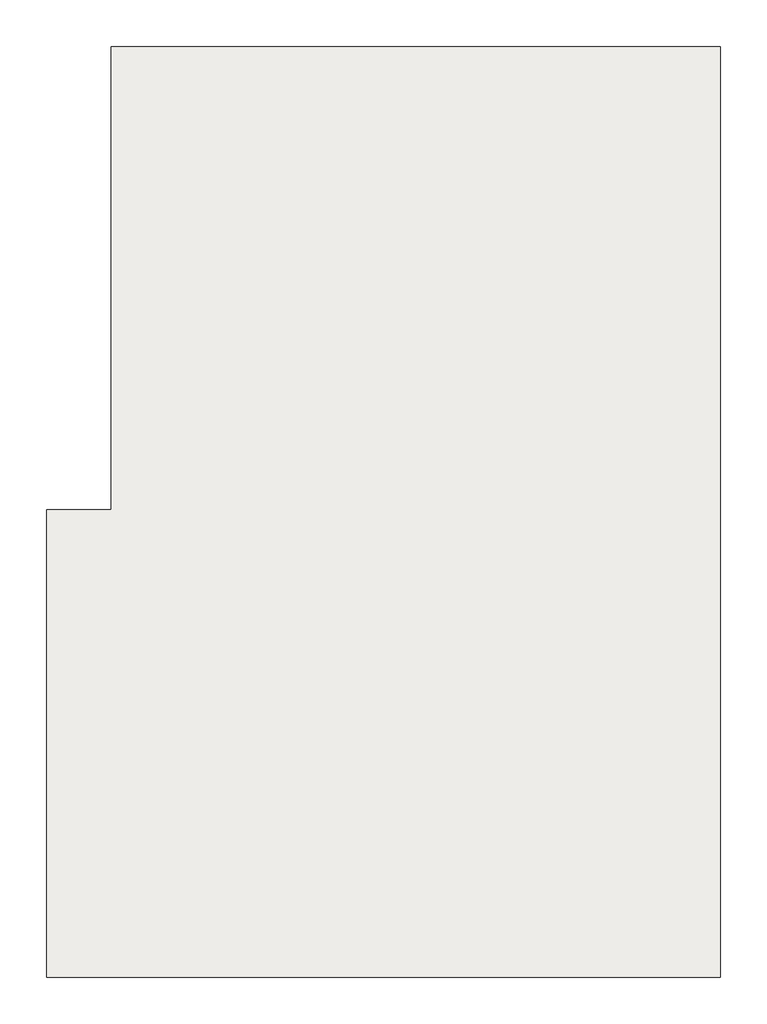
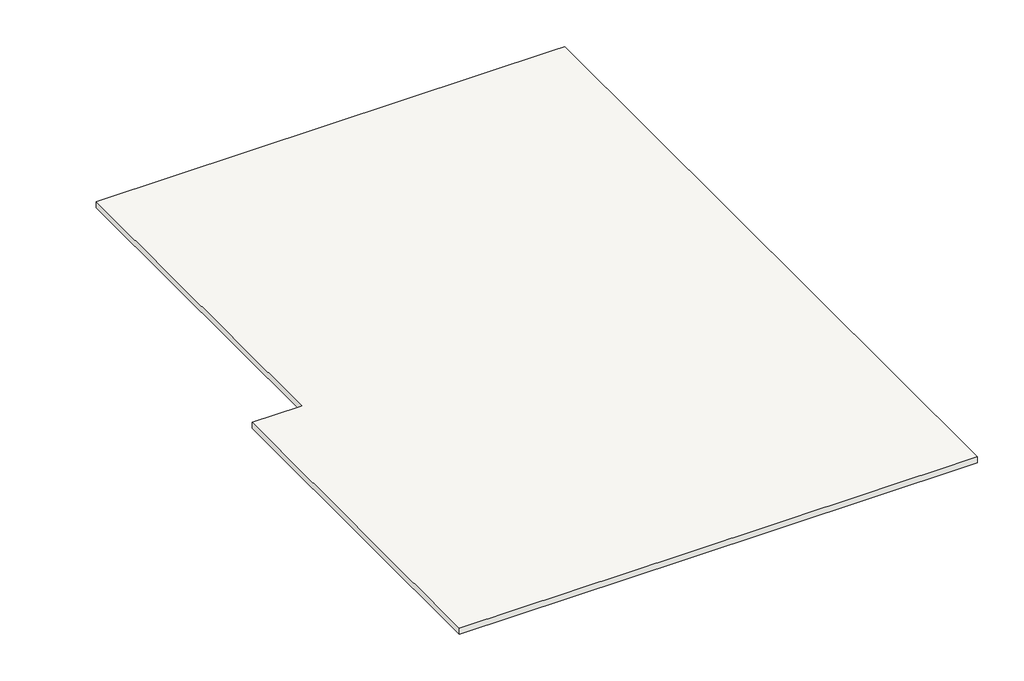
# One storey: 1 slab.
"""IFC4 building model written with IfcOpenShell, lengths in millimetres."""

from ifc_helpers import new_model, si_unit, origin, place, context, project, spatial, faceted_brep, element, save

model = new_model("IFC4")

# Units and contexts
model_context = context("Model", 3, world=origin())
ifc_project = project(units=[si_unit("LENGTHUNIT", "METRE", prefix="MILLI")], contexts=[model_context])

# Site, building, storey
site = spatial("IfcSite", under=ifc_project)
building = spatial("IfcBuilding", under=site)
storey = spatial("IfcBuildingStorey", under=building, Elevation=3657.6)

# Slab
placement = place(None, origin())
element("IfcSlab", 1, ObjectType="6\" 7", at=placement, inside=storey, context=model_context, shape_type="Brep", body=[
    faceted_brep([(6218.7084916, 9466.2935985, 3505.2), (6218.7084916, -8085.1064015, 3505.2), (5990.1084916, -8085.1064015, 3505.2), (-969.7561363, -8085.1064015, 3505.2), (-6494.4004467, -8085.1064015, 3505.2), (-6494.4004467, -4237.1266767, 3505.2), (-6494.4004467, 487.1221373, 3505.2), (-6494.4004467, 728.4221373, 3505.2), (-5287.7561363, 728.4221373, 3505.2), (-5275.0561363, 728.4221373, 3505.2), (-5275.0561363, 9224.9935985, 3505.2), (-5275.0561363, 9466.2935985, 3505.2), (5990.1084916, 9466.2935985, 3505.2), (6218.7084916, 9466.2935985, 3657.6), (5990.1084916, 9466.2935985, 3657.6), (-5275.0561363, 9466.2935985, 3657.6), (-5275.0561363, 9224.9935985, 3657.6), (-5275.0561363, 728.4221373, 3657.6), (-5287.7561363, 728.4221373, 3657.6), (-6494.4004467, 728.4221373, 3657.6), (-6494.4004467, 487.1221373, 3657.6), (-6494.4004467, -4237.1266767, 3657.6), (-6494.4004467, -8085.1064015, 3657.6), (-969.7561363, -8085.1064015, 3657.6), (5990.1084916, -8085.1064015, 3657.6), (6218.7084916, -8085.1064015, 3657.6)], [[[0, 1, 2, 3, 4, 5, 6, 7, 8, 9, 10, 11, 12]], [[13, 14, 15, 16, 17, 18, 19, 20, 21, 22, 23, 24, 25]], [[1, 0, 13, 25]], [[4, 3, 2, 1, 25, 24, 23, 22]], [[0, 12, 11, 15, 14, 13]], [[7, 6, 5, 4, 22, 21, 20, 19]], [[9, 8, 7, 19, 18, 17]], [[11, 10, 9, 17, 16, 15]]]),
])

save(model, "model.ifc")

# Revit data of these elements
# Type "6\" 7"
#   Assembly Code = "B1010"
#   Function = 0
#   Layers, outside or top first: 0' - 6" "INTERIOR TILE" (function 1)
# Element 1 (IfcSlab, "6\" 7")
#   Height Offset From Level = 0' - 0"
#   built-in parameter 1001954 = 1
#   Phase Created = New Construction
#   Materials on its faces: "INTERIOR TILE"
# Materials
#   "INTERIOR TILE": class "Generic", colour RGB 120 120 120, transparency 0, Cost = 0
